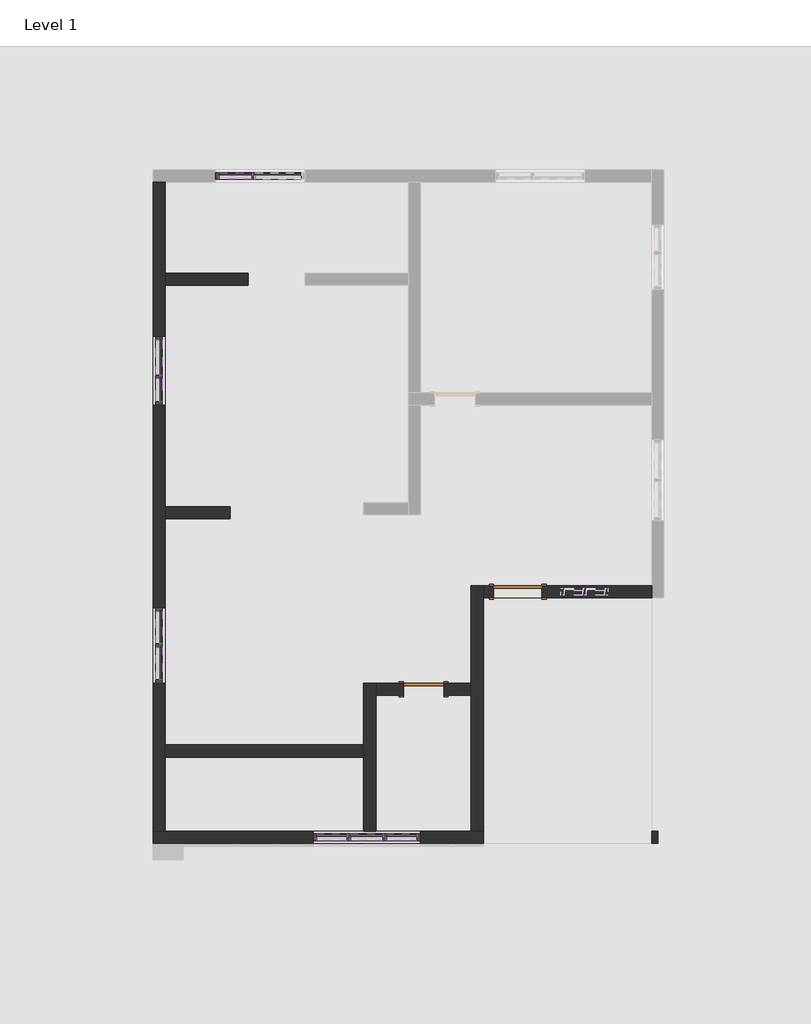
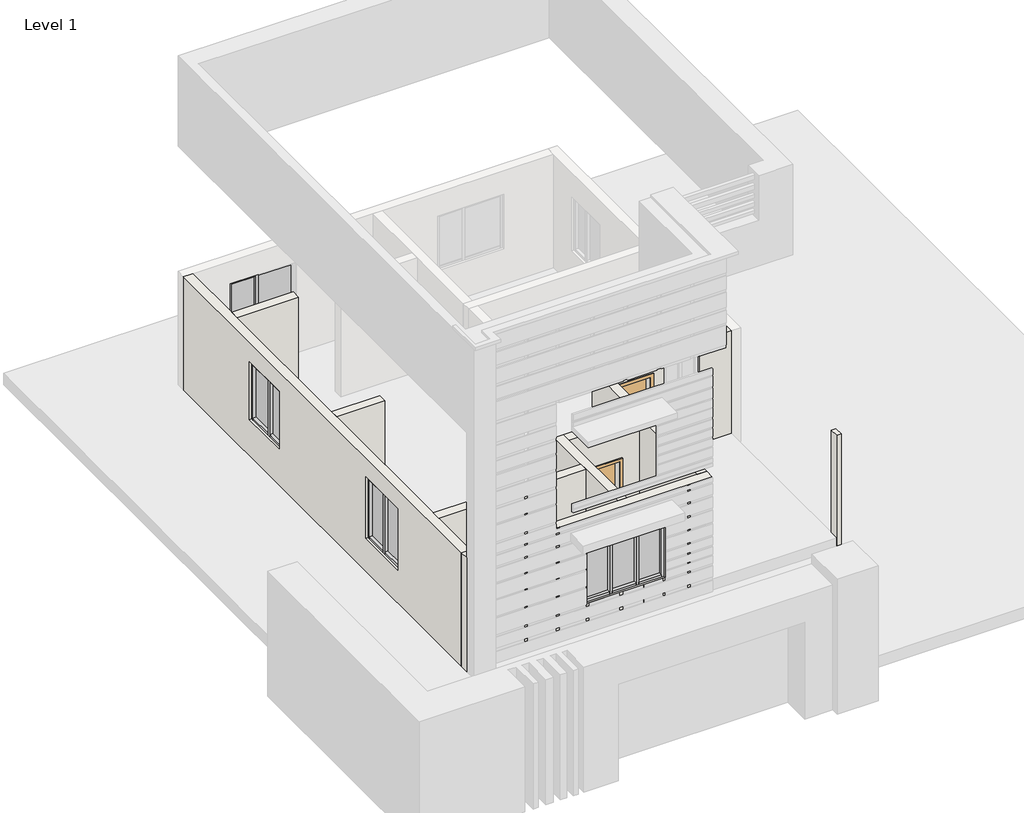
# One storey, part 1 of 2: 29 members, 10 walls, 9 plates, 2 doors.
"""IFC4 building model written with IfcOpenShell, lengths in millimetres."""

from ifc_helpers import new_model, si_unit, frame, origin, origin_with_axes, place, context, project, spatial, polyline, outline, extrude, faceted_brep, transform, mapped, element, save
from components import door_a1484949, door_a90ba1ad, member_830eb86c, member_47bfaf8a, member_eeaa0ee0, member_269e6f2a, member_c33c434a, member_6fb4a552, member_3f0e0172, member_c31ee173, member_024c663a, member_55cf8d67, member_d87774f7, member_b50ca06a, member_72214107, member_f18c796a, system_panel_glazed_8fb17656, system_panel_glazed_f5cea47f, system_panel_glazed_0ce4f10b, system_panel_glazed_3cfdd687, system_panel_glazed_dae3c0ba, system_panel_glazed_60974b7d, system_panel_glazed_18e8007f

model = new_model("IFC4")

# Units and contexts
model_context = context("Model", 3, world=origin())
ifc_project = project(units=[si_unit("LENGTHUNIT", "METRE", prefix="MILLI")], contexts=[model_context])

# Site, building, storey
site = spatial("IfcSite", under=ifc_project)
building = spatial("IfcBuilding", under=site)
storey = spatial("IfcBuildingStorey", under=building, Name="Level 1", Elevation=0.0)

# Doors
placement = place(None, origin())
door_shape = door_a1484949(model_context)
element("IfcDoor", 1, ObjectType="Single-Flush : 30\" x 80\"", at=placement, inside=storey, context=model_context, shape_type="MappedRepresentation", body=[
    mapped(door_shape, transform((-13440.7128107, -10920.6642965, 0.0), x_axis=(1.0, 0.0, 0.0), y_axis=(0.0, 1.0, 0.0), z_axis=(0.0, 0.0, 1.0))),
])
door_2_shape = door_a90ba1ad(model_context)
element("IfcDoor", 2, ObjectType="Single-Flush : 36\" x 84\"", at=placement, inside=storey, context=model_context, shape_type="MappedRepresentation", body=[
    mapped(door_2_shape, transform((-11669.0628107, -9091.8642965, 406.4), x_axis=(-1.0, 0.0, 0.0), y_axis=(0.0, -1.0, 0.0), z_axis=(0.0, 0.0, 1.0))),
])

# Members
member_shape = member_830eb86c(model_context)
element("IfcMember", 3, ObjectType="Rectangular Mullion : 2.5\" x 5\" rectangular", at=placement, inside=storey, context=model_context, shape_type="MappedRepresentation", body=[
    mapped(member_shape, transform((-14875.8128107, -13701.9642965, 2606.1461296), x_axis=(0.0, 0.0, 1.0), y_axis=(0.0, -1.0, 0.0), z_axis=(1.0, 0.0, 0.0))),
])
element("IfcMember", 4, ObjectType="Rectangular Mullion : 2.5\" x 5\" rectangular", at=placement, inside=storey, context=model_context, shape_type="MappedRepresentation", body=[
    mapped(member_shape, transform((-13561.3628107, -13701.9642965, 2606.1461296), x_axis=(0.0, 0.0, 1.0), y_axis=(0.0, -1.0, 0.0), z_axis=(1.0, 0.0, 0.0))),
])
member_2_shape = member_47bfaf8a(model_context)
element("IfcMember", 5, ObjectType="Rectangular Mullion : 2.5\" x 5\" rectangular", at=placement, inside=storey, context=model_context, shape_type="MappedRepresentation", body=[
    mapped(member_2_shape, transform((-14202.7128107, -13701.9642965, 2606.1461296), x_axis=(0.0, 0.0, 1.0), y_axis=(0.0, -1.0, 0.0), z_axis=(1.0, 0.0, 0.0))),
])
element("IfcMember", 6, ObjectType="Rectangular Mullion : 2.5\" x 5\" rectangular", at=placement, inside=storey, context=model_context, shape_type="MappedRepresentation", body=[
    mapped(member_2_shape, transform((-18412.7628107, -10069.7642965, 2535.4608087), x_axis=(0.0, 0.0, 1.0), y_axis=(-1.0, 0.0, 0.0), z_axis=(0.0, -1.0, 0.0))),
])
element("IfcMember", 7, ObjectType="Rectangular Mullion : 2.5\" x 5\" rectangular", at=placement, inside=storey, context=model_context, shape_type="MappedRepresentation", body=[
    mapped(member_2_shape, transform((-18412.7628107, -10742.8642965, 2535.4608087), x_axis=(0.0, 0.0, 1.0), y_axis=(-1.0, 0.0, 0.0), z_axis=(0.0, -1.0, 0.0))),
])
member_3_shape = member_eeaa0ee0(model_context)
element("IfcMember", 8, ObjectType="Rectangular Mullion : 2.5\" x 5\" rectangular", at=placement, inside=storey, context=model_context, shape_type="MappedRepresentation", body=[
    mapped(member_3_shape, transform((-14844.0628107, -13701.9642965, 763.0716334), x_axis=(1.0, 0.0, 0.0), y_axis=(0.0, -1.0, 0.0), z_axis=(0.0, 0.0, -1.0))),
])
element("IfcMember", 9, ObjectType="Rectangular Mullion : 2.5\" x 5\" rectangular", at=placement, inside=storey, context=model_context, shape_type="MappedRepresentation", body=[
    mapped(member_3_shape, transform((-14170.9628107, -13701.9642965, 763.0716334), x_axis=(1.0, 0.0, 0.0), y_axis=(0.0, -1.0, 0.0), z_axis=(0.0, 0.0, -1.0))),
])
element("IfcMember", 10, ObjectType="Rectangular Mullion : 2.5\" x 5\" rectangular", at=placement, inside=storey, context=model_context, shape_type="MappedRepresentation", body=[
    mapped(member_shape, transform((-14139.2128107, -13701.9642965, 763.0716334), x_axis=(0.0, 0.0, -1.0), y_axis=(0.0, -1.0, 0.0), z_axis=(-1.0, 0.0, 0.0))),
])
element("IfcMember", 11, ObjectType="Rectangular Mullion : 2.5\" x 5\" rectangular", at=placement, inside=storey, context=model_context, shape_type="MappedRepresentation", body=[
    mapped(member_shape, transform((-15453.6628107, -13701.9642965, 763.0716334), x_axis=(0.0, 0.0, -1.0), y_axis=(0.0, -1.0, 0.0), z_axis=(-1.0, 0.0, 0.0))),
])
element("IfcMember", 12, ObjectType="Rectangular Mullion : 2.5\" x 5\" rectangular", at=placement, inside=storey, context=model_context, shape_type="MappedRepresentation", body=[
    mapped(member_2_shape, transform((-14812.3128107, -13701.9642965, 763.0716334), x_axis=(0.0, 0.0, -1.0), y_axis=(0.0, -1.0, 0.0), z_axis=(-1.0, 0.0, 0.0))),
])
element("IfcMember", 13, ObjectType="Rectangular Mullion : 2.5\" x 5\" rectangular", at=placement, inside=storey, context=model_context, shape_type="MappedRepresentation", body=[
    mapped(member_2_shape, transform((-18412.7628107, -10133.2642965, 888.5243078), x_axis=(0.0, 0.0, -1.0), y_axis=(-1.0, 0.0, 0.0), z_axis=(0.0, 1.0, 0.0))),
])
element("IfcMember", 14, ObjectType="Rectangular Mullion : 2.5\" x 5\" rectangular", at=placement, inside=storey, context=model_context, shape_type="MappedRepresentation", body=[
    mapped(member_2_shape, transform((-18412.7628107, -9460.1642965, 888.5243078), x_axis=(0.0, 0.0, -1.0), y_axis=(-1.0, 0.0, 0.0), z_axis=(0.0, 1.0, 0.0))),
])
member_4_shape = member_269e6f2a(model_context)
element("IfcMember", 15, ObjectType="Rectangular Mullion : 2.5\" x 5\" rectangular", at=placement, inside=storey, context=model_context, shape_type="MappedRepresentation", body=[
    mapped(member_4_shape, transform((-15517.1628107, -13701.9642965, 2606.1461296), x_axis=(-1.0, 0.0, 0.0), y_axis=(0.0, -1.0, 0.0), z_axis=(0.0, 0.0, 1.0))),
])
element("IfcMember", 16, ObjectType="Rectangular Mullion : 2.5\" x 5\" rectangular", at=placement, inside=storey, context=model_context, shape_type="MappedRepresentation", body=[
    mapped(member_4_shape, transform((-13497.8628107, -13701.9642965, 763.0716334), x_axis=(1.0, 0.0, 0.0), y_axis=(0.0, -1.0, 0.0), z_axis=(0.0, 0.0, -1.0))),
])
member_5_shape = member_c33c434a(model_context)
element("IfcMember", 17, ObjectType="Rectangular Mullion : 2.5\" x 5\" rectangular", at=placement, inside=storey, context=model_context, shape_type="MappedRepresentation", body=[
    mapped(member_5_shape, transform((-18412.7628107, -4354.7642965, 971.9632466), x_axis=(0.0, 0.0, -1.0), y_axis=(-1.0, 0.0, 0.0), z_axis=(0.0, 1.0, 0.0))),
])
element("IfcMember", 18, ObjectType="Rectangular Mullion : 2.5\" x 5\" rectangular", at=placement, inside=storey, context=model_context, shape_type="MappedRepresentation", body=[
    mapped(member_5_shape, transform((-18412.7628107, -5021.5142965, 2516.3699232), x_axis=(0.0, 0.0, 1.0), y_axis=(-1.0, 0.0, 0.0), z_axis=(0.0, -1.0, 0.0))),
])
member_6_shape = member_6fb4a552(model_context)
element("IfcMember", 19, ObjectType="Rectangular Mullion : 2.5\" x 5\" rectangular", at=placement, inside=storey, context=model_context, shape_type="MappedRepresentation", body=[
    mapped(member_6_shape, transform((-18412.7628107, -5085.0142965, 971.9632466), x_axis=(0.0, 0.0, -1.0), y_axis=(-1.0, 0.0, 0.0), z_axis=(0.0, 1.0, 0.0))),
])
element("IfcMember", 20, ObjectType="Rectangular Mullion : 2.5\" x 5\" rectangular", at=placement, inside=storey, context=model_context, shape_type="MappedRepresentation", body=[
    mapped(member_6_shape, transform((-18412.7628107, -5523.1642965, 2516.3699232), x_axis=(0.0, 0.0, 1.0), y_axis=(-1.0, 0.0, 0.0), z_axis=(0.0, -1.0, 0.0))),
])
member_7_shape = member_3f0e0172(model_context)
element("IfcMember", 21, ObjectType="Rectangular Mullion : 2.5\" x 5\" rectangular", at=placement, inside=storey, context=model_context, shape_type="MappedRepresentation", body=[
    mapped(member_7_shape, transform((-16666.5128107, -1281.3642965, 2436.257419), x_axis=(0.0, 0.0, 1.0), y_axis=(0.0, -1.0, 0.0), z_axis=(1.0, 0.0, 0.0))),
])
member_8_shape = member_c31ee173(model_context)
element("IfcMember", 22, ObjectType="Rectangular Mullion : 2.5\" x 5\" rectangular", at=placement, inside=storey, context=model_context, shape_type="MappedRepresentation", body=[
    mapped(member_8_shape, transform((-16634.7628107, -1281.3642965, 1057.7597182), x_axis=(1.0, 0.0, 0.0), y_axis=(0.0, -1.0, 0.0), z_axis=(0.0, 0.0, -1.0))),
])
member_9_shape = member_024c663a(model_context)
element("IfcMember", 23, ObjectType="Rectangular Mullion : 2.5\" x 5\" rectangular", at=placement, inside=storey, context=model_context, shape_type="MappedRepresentation", body=[
    mapped(member_9_shape, transform((-16603.0128107, -1281.3642965, 1057.7597182), x_axis=(0.0, 0.0, -1.0), y_axis=(0.0, -1.0, 0.0), z_axis=(-1.0, 0.0, 0.0))),
])
element("IfcMember", 24, ObjectType="Rectangular Mullion : 2.5\" x 5\" rectangular", at=placement, inside=storey, context=model_context, shape_type="MappedRepresentation", body=[
    mapped(member_7_shape, transform((-17282.4628107, -1281.3642965, 1057.7597182), x_axis=(0.0, 0.0, -1.0), y_axis=(0.0, -1.0, 0.0), z_axis=(-1.0, 0.0, 0.0))),
])
member_10_shape = member_55cf8d67(model_context)
element("IfcMember", 25, ObjectType="Rectangular Mullion : 2.5\" x 5\" rectangular", at=placement, inside=storey, context=model_context, shape_type="MappedRepresentation", body=[
    mapped(member_10_shape, transform((-17345.9628107, -1281.3642965, 2436.257419), x_axis=(-1.0, 0.0, 0.0), y_axis=(0.0, -1.0, 0.0), z_axis=(0.0, 0.0, 1.0))),
])
member_11_shape = member_d87774f7(model_context)
element("IfcMember", 26, ObjectType="Rectangular Mullion : 2.5\" x 5\" rectangular", at=placement, inside=storey, context=model_context, shape_type="MappedRepresentation", body=[
    mapped(member_11_shape, transform((-18412.7628107, -5053.2642965, 971.9632466), x_axis=(0.0, -1.0, 0.0), y_axis=(-1.0, 0.0, 0.0), z_axis=(0.0, 0.0, -1.0))),
])
member_12_shape = member_b50ca06a(model_context)
element("IfcMember", 27, ObjectType="Rectangular Mullion : 2.5\" x 5\" rectangular", at=placement, inside=storey, context=model_context, shape_type="MappedRepresentation", body=[
    mapped(member_12_shape, transform((-18412.7628107, -5586.6642965, 971.9632466), x_axis=(0.0, -1.0, 0.0), y_axis=(-1.0, 0.0, 0.0), z_axis=(0.0, 0.0, -1.0))),
])
element("IfcMember", 28, ObjectType="Rectangular Mullion : 2.5\" x 5\" rectangular", at=placement, inside=storey, context=model_context, shape_type="MappedRepresentation", body=[
    mapped(member_12_shape, transform((-18412.7628107, -4291.2642965, 2516.3699232), x_axis=(0.0, 1.0, 0.0), y_axis=(-1.0, 0.0, 0.0), z_axis=(0.0, 0.0, 1.0))),
])
member_13_shape = member_72214107(model_context)
element("IfcMember", 29, ObjectType="Rectangular Mullion : 2.5\" x 5\" rectangular", at=placement, inside=storey, context=model_context, shape_type="MappedRepresentation", body=[
    mapped(member_13_shape, transform((-18412.7628107, -10101.5142965, 888.5243078), x_axis=(0.0, -1.0, 0.0), y_axis=(-1.0, 0.0, 0.0), z_axis=(0.0, 0.0, -1.0))),
])
member_14_shape = member_f18c796a(model_context)
element("IfcMember", 30, ObjectType="Rectangular Mullion : 2.5\" x 5\" rectangular", at=placement, inside=storey, context=model_context, shape_type="MappedRepresentation", body=[
    mapped(member_14_shape, transform((-18412.7628107, -9396.6642965, 2535.4608087), x_axis=(0.0, 1.0, 0.0), y_axis=(-1.0, 0.0, 0.0), z_axis=(0.0, 0.0, 1.0))),
])
element("IfcMember", 31, ObjectType="Rectangular Mullion : 2.5\" x 5\" rectangular", at=placement, inside=storey, context=model_context, shape_type="MappedRepresentation", body=[
    mapped(member_14_shape, transform((-18412.7628107, -10806.3642965, 888.5243078), x_axis=(0.0, -1.0, 0.0), y_axis=(-1.0, 0.0, 0.0), z_axis=(0.0, 0.0, -1.0))),
])

# Plates
system_panel_glazed_shape = system_panel_glazed_8fb17656(model_context)
element("IfcPlate", 32, ObjectType="System Panel : Glazed", at=placement, inside=storey, context=model_context, shape_type="MappedRepresentation", body=[
    mapped(system_panel_glazed_shape, transform((-15164.7378107, -13701.9642965, 826.5716334), x_axis=(1.0, 0.0, 0.0), y_axis=(0.0, 1.0, 0.0), z_axis=(0.0, 0.0, 1.0))),
])
element("IfcPlate", 33, ObjectType="System Panel : Glazed", at=placement, inside=storey, context=model_context, shape_type="MappedRepresentation", body=[
    mapped(system_panel_glazed_shape, transform((-13850.2878107, -13701.9642965, 826.5716334), x_axis=(1.0, 0.0, 0.0), y_axis=(0.0, 1.0, 0.0), z_axis=(0.0, 0.0, 1.0))),
])
system_panel_glazed_2_shape = system_panel_glazed_f5cea47f(model_context)
element("IfcPlate", 34, ObjectType="System Panel : Glazed", at=placement, inside=storey, context=model_context, shape_type="MappedRepresentation", body=[
    mapped(system_panel_glazed_2_shape, transform((-14507.5128107, -13701.9642965, 826.5716334), x_axis=(1.0, 0.0, 0.0), y_axis=(0.0, 1.0, 0.0), z_axis=(0.0, 0.0, 1.0))),
])
system_panel_glazed_3_shape = system_panel_glazed_0ce4f10b(model_context)
element("IfcPlate", 35, ObjectType="System Panel : Glazed", at=placement, inside=storey, context=model_context, shape_type="MappedRepresentation", body=[
    mapped(system_panel_glazed_3_shape, transform((-16974.4878107, -1281.3642965, 1121.2597182), x_axis=(1.0, 0.0, 0.0), y_axis=(0.0, 1.0, 0.0), z_axis=(0.0, 0.0, 1.0))),
])
system_panel_glazed_4_shape = system_panel_glazed_3cfdd687(model_context)
element("IfcPlate", 36, ObjectType="System Panel : Glazed", at=placement, inside=storey, context=model_context, shape_type="MappedRepresentation", body=[
    mapped(system_panel_glazed_4_shape, transform((-16168.0378107, -1281.3642965, 1121.2597182), x_axis=(1.0, 0.0, 0.0), y_axis=(0.0, 1.0, 0.0), z_axis=(0.0, 0.0, 1.0))),
])
system_panel_glazed_5_shape = system_panel_glazed_dae3c0ba(model_context)
element("IfcPlate", 37, ObjectType="System Panel : Glazed", at=placement, inside=storey, context=model_context, shape_type="MappedRepresentation", body=[
    mapped(system_panel_glazed_5_shape, transform((-18412.7628107, -4688.1392965, 1035.4632466), x_axis=(0.0, -1.0, 0.0), y_axis=(1.0, 0.0, 0.0), z_axis=(0.0, 0.0, 1.0))),
])
system_panel_glazed_6_shape = system_panel_glazed_60974b7d(model_context)
element("IfcPlate", 38, ObjectType="System Panel : Glazed", at=placement, inside=storey, context=model_context, shape_type="MappedRepresentation", body=[
    mapped(system_panel_glazed_6_shape, transform((-18412.7628107, -5304.0892965, 1035.4632466), x_axis=(0.0, -1.0, 0.0), y_axis=(1.0, 0.0, 0.0), z_axis=(0.0, 0.0, 1.0))),
])
system_panel_glazed_7_shape = system_panel_glazed_18e8007f(model_context)
element("IfcPlate", 39, ObjectType="System Panel : Glazed", at=placement, inside=storey, context=model_context, shape_type="MappedRepresentation", body=[
    mapped(system_panel_glazed_7_shape, transform((-18412.7628107, -9764.9642965, 952.0243078), x_axis=(0.0, -1.0, 0.0), y_axis=(1.0, 0.0, 0.0), z_axis=(0.0, 0.0, 1.0))),
])
element("IfcPlate", 40, ObjectType="System Panel : Glazed", at=placement, inside=storey, context=model_context, shape_type="MappedRepresentation", body=[
    mapped(system_panel_glazed_7_shape, transform((-18412.7628107, -10438.0642965, 952.0243078), x_axis=(0.0, -1.0, 0.0), y_axis=(1.0, 0.0, 0.0), z_axis=(0.0, 0.0, 1.0))),
])

# Walls
element("IfcWall", 41, ObjectType="9\"", at=placement, inside=storey, context=model_context, shape_type="Brep", body=[
    faceted_brep([(-18527.0628107, -13816.2642965, 0.0), (-12316.7628107, -13816.2642965, 0.0), (-12316.7628107, -13816.2642965, 3048.0), (-18527.0628107, -13816.2642965, 3048.0), (-15517.1628107, -13816.2642965, 763.0716334), (-15517.1628107, -13816.2642965, 2606.1461296), (-13497.8628107, -13816.2642965, 2606.1461296), (-13497.8628107, -13816.2642965, 763.0716334), (-12316.7628107, -13587.6642965, 0.0), (-12545.3628107, -13587.6642965, 0.0), (-14336.0628107, -13587.6642965, 0.0), (-14564.6628107, -13587.6642965, 0.0), (-18298.4628107, -13587.6642965, 0.0), (-18527.0628107, -13587.6642965, 0.0), (-18527.0628107, -13587.6642965, 3048.0), (-18298.4628107, -13587.6642965, 3048.0), (-14564.6628107, -13587.6642965, 3048.0), (-14336.0628107, -13587.6642965, 3048.0), (-12545.3628107, -13587.6642965, 3048.0), (-12316.7628107, -13587.6642965, 3048.0), (-15517.1628107, -13587.6642965, 2606.1461296), (-15517.1628107, -13587.6642965, 763.0716334), (-13497.8628107, -13587.6642965, 763.0716334), (-13497.8628107, -13587.6642965, 2606.1461296)], [[[0, 1, 2, 3], [4, 5, 6, 7]], [[8, 9, 10, 11, 12, 13, 14, 15, 16, 17, 18, 19], [20, 21, 22, 23]], [[1, 0, 13, 12, 11, 10, 9, 8]], [[2, 1, 8, 19]], [[3, 2, 19, 18, 17, 16, 15, 14]], [[0, 3, 14, 13]], [[4, 21, 20, 5]], [[5, 20, 23, 6]], [[6, 23, 22, 7]], [[21, 4, 7, 22]]]),
])
element("IfcWall", 42, ObjectType="9\"", at=placement, inside=storey, context=model_context, shape_type="Brep", body=[
    faceted_brep([(-18527.0628107, -1395.6642965, 0.0), (-18527.0628107, -13587.6642965, 0.0), (-18527.0628107, -13587.6642965, 3048.0), (-18527.0628107, -1395.6642965, 3048.0), (-18527.0628107, -4291.2642965, 971.9632466), (-18527.0628107, -4291.2642965, 2516.3699232), (-18527.0628107, -5586.6642965, 2516.3699232), (-18527.0628107, -5586.6642965, 971.9632466), (-18527.0628107, -9396.6642965, 888.5243078), (-18527.0628107, -9396.6642965, 2535.4608087), (-18527.0628107, -10806.3642965, 2535.4608087), (-18527.0628107, -10806.3642965, 888.5243078), (-18298.4628107, -13587.6642965, 0.0), (-18298.4628107, -12197.0142965, 0.0), (-18298.4628107, -11968.4142965, 0.0), (-18298.4628107, -7720.2642965, 0.0), (-18298.4628107, -7491.6642965, 0.0), (-18298.4628107, -3338.7642965, 0.0), (-18298.4628107, -3110.1642965, 0.0), (-18298.4628107, -1395.6642965, 0.0), (-18298.4628107, -1395.6642965, 3048.0), (-18298.4628107, -3110.1642965, 3048.0), (-18298.4628107, -3338.7642965, 3048.0), (-18298.4628107, -7491.6642965, 3048.0), (-18298.4628107, -7720.2642965, 3048.0), (-18298.4628107, -11968.4142965, 3048.0), (-18298.4628107, -12197.0142965, 3048.0), (-18298.4628107, -13587.6642965, 3048.0), (-18298.4628107, -4291.2642965, 2516.3699232), (-18298.4628107, -4291.2642965, 971.9632466), (-18298.4628107, -5586.6642965, 971.9632466), (-18298.4628107, -5586.6642965, 2516.3699232), (-18298.4628107, -9396.6642965, 2535.4608087), (-18298.4628107, -9396.6642965, 888.5243078), (-18298.4628107, -10806.3642965, 888.5243078), (-18298.4628107, -10806.3642965, 2535.4608087)], [[[0, 1, 2, 3], [4, 5, 6, 7], [8, 9, 10, 11]], [[12, 13, 14, 15, 16, 17, 18, 19, 20, 21, 22, 23, 24, 25, 26, 27], [28, 29, 30, 31], [32, 33, 34, 35]], [[1, 0, 19, 18, 17, 16, 15, 14, 13, 12]], [[3, 2, 27, 26, 25, 24, 23, 22, 21, 20]], [[0, 3, 20, 19]], [[2, 1, 12, 27]], [[4, 29, 28, 5]], [[5, 28, 31, 6]], [[6, 31, 30, 7]], [[29, 4, 7, 30]], [[8, 33, 32, 9]], [[9, 32, 35, 10]], [[34, 11, 10, 35]], [[33, 8, 11, 34]]]),
])
element("IfcWall", 43, ObjectType="9\"", at=placement, inside=storey, context=model_context, shape_type="Brep", body=[
    faceted_brep([(-12316.7628107, -13587.6642965, 0.0), (-12316.7628107, -9206.1642965, 0.0), (-12316.7628107, -8977.5642965, 0.0), (-12316.7628107, -8977.5642965, 3048.0), (-12316.7628107, -9206.1642965, 3048.0), (-12316.7628107, -13587.6642965, 3048.0), (-12545.3628107, -13587.6642965, 0.0), (-12545.3628107, -13587.6642965, 3048.0), (-12545.3628107, -11034.9642965, 3048.0), (-12545.3628107, -10806.3642965, 3048.0), (-12545.3628107, -8977.5642965, 3048.0), (-12545.3628107, -8977.5642965, 0.0), (-12545.3628107, -10806.3642965, 0.0), (-12545.3628107, -11034.9642965, 0.0)], [[[0, 1, 2, 3, 4, 5]], [[6, 7, 8, 9, 10, 11, 12, 13]], [[2, 1, 0, 6, 13, 12, 11]], [[5, 4, 3, 10, 9, 8, 7]], [[0, 5, 7, 6]], [[3, 2, 11, 10]]]),
])
element("IfcWall", 44, ObjectType="9\"", at=placement, inside=storey, context=model_context, shape_type="SweptSolid", body=[
    extrude(outline(polyline([(0.0, -12316.7628107), (0.0, -9154.4628107), (3048.0, -9154.4628107), (3048.0, -12316.7628107), (0.0, -12316.7628107)]), holes=[polyline([(406.4, -11211.8628107), (406.4, -12126.2628107), (2540.0, -12126.2628107), (2540.0, -11211.8628107), (406.4, -11211.8628107)]), polyline([(1249.7277266, -10856.2628107), (2736.7021457, -10856.2628107), (2736.7021457, -9973.6128107), (1249.7277266, -9973.6128107), (1249.7277266, -10856.2628107)])]), frame((0.0, -9206.1642965, 0.0), z_axis=(0.0, 1.0, 0.0), x_axis=(0.0, 0.0, 1.0)), (0.0, 0.0, 1.0), 228.6),
])
element("IfcWall", 45, ObjectType="9\"", at=placement, inside=storey, context=model_context, shape_type="Brep", body=[
    faceted_brep([(-14336.0628107, -13587.6642965, 0.0), (-14336.0628107, -11034.9642965, 0.0), (-14336.0628107, -10806.3642965, 0.0), (-14336.0628107, -10806.3642965, 3048.0), (-14336.0628107, -11034.9642965, 3048.0), (-14336.0628107, -13587.6642965, 3048.0), (-14564.6628107, -13587.6642965, 0.0), (-14564.6628107, -13587.6642965, 3048.0), (-14564.6628107, -12197.0142965, 3048.0), (-14564.6628107, -11968.4142965, 3048.0), (-14564.6628107, -10806.3642965, 3048.0), (-14564.6628107, -10806.3642965, 0.0), (-14564.6628107, -11968.4142965, 0.0), (-14564.6628107, -12197.0142965, 0.0)], [[[0, 1, 2, 3, 4, 5]], [[6, 7, 8, 9, 10, 11, 12, 13]], [[2, 1, 0, 6, 13, 12, 11]], [[5, 4, 3, 10, 9, 8, 7]], [[0, 5, 7, 6]], [[3, 2, 11, 10]]]),
])
element("IfcWall", 46, ObjectType="9\"", at=placement, inside=storey, context=model_context, shape_type="SweptSolid", body=[
    extrude(outline(polyline([(2032.0, -13059.7128107), (0.0, -13059.7128107), (0.0, -12545.3628107), (3048.0, -12545.3628107), (3048.0, -14336.0628107), (0.0, -14336.0628107), (0.0, -13821.7128107), (2032.0, -13821.7128107), (2032.0, -13059.7128107)])), frame((0.0, -11034.9642965, 0.0), z_axis=(0.0, 1.0, 0.0), x_axis=(0.0, 0.0, 1.0)), (0.0, 0.0, 1.0), 228.6),
])
element("IfcWall", 47, ObjectType="9\"", at=placement, inside=storey, context=model_context, shape_type="SweptSolid", body=[
    extrude(outline(polyline([(-18298.4628107, -11968.4142965), (-14564.6628107, -11968.4142965), (-14564.6628107, -12197.0142965), (-18298.4628107, -12197.0142965), (-18298.4628107, -11968.4142965)])), origin_with_axes(), (0.0, 0.0, 1.0), 3048.0),
])
element("IfcWall", 48, ObjectType="9\"", at=placement, inside=storey, context=model_context, shape_type="SweptSolid", body=[
    extrude(outline(polyline([(-16736.3628107, -3338.7642965), (-18298.4628107, -3338.7642965), (-18298.4628107, -3110.1642965), (-16736.3628107, -3110.1642965), (-16736.3628107, -3338.7642965)])), origin_with_axes(), (0.0, 0.0, 1.0), 3048.0),
])
element("IfcWall", 49, ObjectType="9\"", at=placement, inside=storey, context=model_context, shape_type="SweptSolid", body=[
    extrude(outline(polyline([(-17079.2628107, -7720.2642965), (-18298.4628107, -7720.2642965), (-18298.4628107, -7491.6642965), (-17079.2628107, -7491.6642965), (-17079.2628107, -7720.2642965)])), origin_with_axes(), (0.0, 0.0, 1.0), 3048.0),
])
element("IfcWall", 50, ObjectType="9\"", at=placement, inside=storey, context=model_context, shape_type="SweptSolid", body=[
    extrude(outline(polyline([(-9040.1628107, -13816.2642965), (-9154.4628107, -13816.2642965), (-9154.4628107, -13587.6642965), (-9040.1628107, -13587.6642965), (-9040.1628107, -13816.2642965)])), origin_with_axes(), (0.0, 0.0, 1.0), 3048.0),
])

save(model, "model.ifc")

# Revit data of these elements
# Type "Single-Flush : 30\" x 80\""
#   Type Mark = "5"
#   Construction Type Id = "MDOOR"
#   Assembly Code = "C1020"
#   Analytic Construction = "Metal"
#   Thickness = 0' - 2"
#   Heat Transfer Coefficient (U) = 0.651978 BTU/(h·ft²·°F)
#   Height = 6' - 8"
#   Trim Projection Ext = 0' - 1"
#   Trim Projection Int = 0' - 1"
#   Trim Width = 0' - 3"
#   Width = 2' - 6"
#   Define Thermal Properties by = 1
#   Define Thermal Properties by = 1
#   Door Material = Door - Panel
#   Frame Material = Door - Frame
#   Visual Light Transmittance = 0
#   Solar Heat Gain Coefficient = 0
#   Function = (empty or 0)
#   Wall Closure = (empty or 0)
# Type "Single-Flush : 36\" x 84\""
#   Type Mark = "1"
#   Construction Type Id = "MDOOR"
#   Assembly Code = "C1020"
#   Analytic Construction = "Metal"
#   Thickness = 0' - 2"
#   Heat Transfer Coefficient (U) = 0.651978 BTU/(h·ft²·°F)
#   Height = 7' - 0"
#   Trim Projection Ext = 0' - 1"
#   Trim Projection Int = 0' - 1"
#   Trim Width = 0' - 3"
#   Width = 3' - 0"
#   Define Thermal Properties by = 1
#   Define Thermal Properties by = 1
#   Door Material = Door - Panel
#   Frame Material = Door - Frame
#   Visual Light Transmittance = 0
#   Solar Heat Gain Coefficient = 0
#   Function = (empty or 0)
#   Wall Closure = (empty or 0)
# Type "Rectangular Mullion : 2.5\" x 5\" rectangular"
#   built-in parameter 1007304 = 0.416667 (stored number, unit not read)
#   built-in parameter 1007301 = 0.104167 (stored number, unit not read)
#   built-in parameter 1007300 = 0.104167 (stored number, unit not read)
# Type "System Panel : Glazed"
#   Construction Type Id = "GSP4R"
#   Analytic Construction = "1/8 in Pilkington single glazing"
#   Visual Light Transmittance = 0.9
#   Solar Heat Gain Coefficient = 0.86
#   Heat Transfer Coefficient (U) = 1.18115 BTU/(h·ft²·°F)
#   Define Thermal Properties by = 1
# Type "9\""
#   Assembly Code = "B2010"
#   Layers, outside or top first: 0' - 9" no material (function 1)
# Element 1 (IfcDoor, "Single-Flush : 30\" x 80\"")
#   Phase Created = New Construction
#   Materials on its faces: "Door - Frame", "Door - Panel"
# Element 2 (IfcDoor, "Single-Flush : 36\" x 84\"")
#   Phase Created = New Construction
#   Materials on its faces: "Door - Frame", "Door - Panel"
# Elements 3, 4, 5, 6, 7, 8, 9, 10, 11, 12, 13, 14, 15, 16, 17, 18, 19, 20, 21, 22, 23, 24, 25, 26, 27, 28, 29, 30, 31 (IfcMember, "Rectangular Mullion : 2.5\" x 5\" rectangular")
#   Phase Created = New Construction
#   Materials on its faces: "Aluminum"
# Elements 32, 33, 34, 35, 36, 37, 38, 39, 40 (IfcPlate, "System Panel : Glazed")
#   Phase Created = New Construction
#   Materials on its faces: "Glass"
# Elements 41, 42, 43, 44, 45, 46, 47, 48, 49, 50 (IfcWall, "9\"")
#   Top Offset = 0' - 0"
#   Base Offset = 0' - 0"
#   Unconnected Height = 10' - 0"
#   wall height = 10' - 0"
#   Phase Created = New Construction
#   Base Constraint = Level 1
#   Materials on its faces: "Default Wall"
# Materials
#   "Door - Panel": class "Wood", colour RGB 210 159 95, transparency 0, Cost = 0
#   "Door - Frame": colour RGB 118 70 51, transparency 0, Cost = 0
#   "Aluminum": class "Metal", colour RGB 247 247 247, transparency 0, Description = "Aluminum 6061", Cost = 0
#   "Glass": class "Glass", colour RGB 0 128 192, transparency 0.75, Description = "Soda Lime Glass", Cost = 0
#   "Default Wall": colour RGB 128 128 128, transparency 0, Cost = 0
